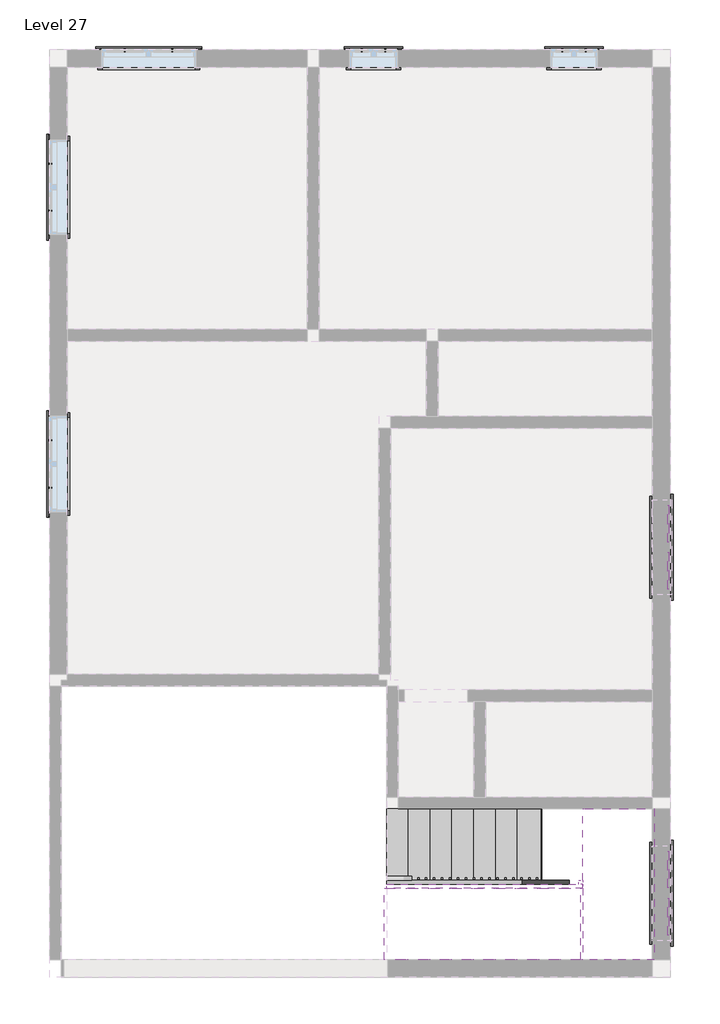
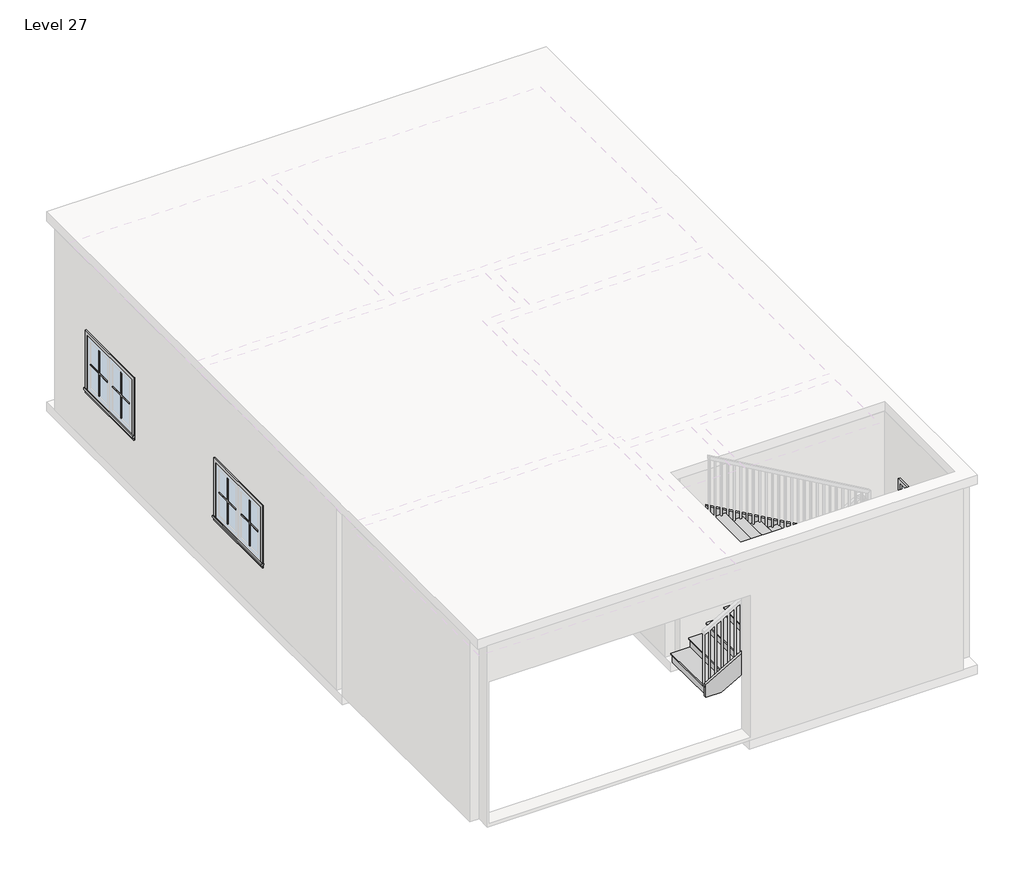
# One storey, part 3 of 3: 44 proxies, 6 members, 4 stair flights, 2 slabs.
"""IFC4 building model written with IfcOpenShell, lengths in millimetres."""

from ifc_helpers import new_model, si_unit, frame, origin, place, context, project, spatial, polyline, outline, extrude, transform, mapped, element, save
from components import muntin_pattern_2x2_muntin_pattern_2x2_2357e71d, muntin_pattern_2x2_muntin_pattern_2x2_302d8f29, muntin_pattern_2x2_muntin_pattern_2x2_53152e2c, muntin_pattern_2x2_muntin_pattern_2x2_e8f3e573, trim_window_exterior_flat_with_sill_c4e67c73, trim_window_exterior_flat_with_sill_a665a915, trim_window_interior_flat_picture_frame_cf1733af, trim_window_interior_flat_picture_frame_d485c387, non_monolithic_landing_8fd7ddd1, stair_flight_a002e3d3, stair_flight_1fb61bbc

model = new_model("IFC4")

# Units and contexts
model_context = context("Model", 3, world=origin())
ifc_project = project(units=[si_unit("LENGTHUNIT", "METRE", prefix="MILLI")], contexts=[model_context])

# Site, building, storey
site = spatial("IfcSite", under=ifc_project)
building = spatial("IfcBuilding", under=site)
storey = spatial("IfcBuildingStorey", under=building, Name="Level 27", Elevation=22402.8)

# Proxies
placement = place(None, origin())
muntin_pattern_2x2_muntin_pattern_2x2_shape = muntin_pattern_2x2_muntin_pattern_2x2_2357e71d(model_context)
element("IfcBuildingElementProxy", 1, Name="Muntin Pattern_2x2 : Muntin Pattern_2x2", ObjectType="Muntin Pattern_2x2 : Muntin Pattern_2x2", at=placement, inside=storey, context=model_context, shape_type="MappedRepresentation", body=[
    mapped(muntin_pattern_2x2_muntin_pattern_2x2_shape, transform((-4942.3279463, 5897.3080275, 23387.05), x_axis=(1.0, 0.0, 0.0), y_axis=(0.0, 1.0, 0.0), z_axis=(0.0, 0.0, 1.0))),
])
element("IfcBuildingElementProxy", 2, Name="Muntin Pattern_2x2 : Muntin Pattern_2x2", ObjectType="Muntin Pattern_2x2 : Muntin Pattern_2x2", at=placement, inside=storey, context=model_context, shape_type="MappedRepresentation", body=[
    mapped(muntin_pattern_2x2_muntin_pattern_2x2_shape, transform((-5899.5904463, 3838.3205275, 23387.05), x_axis=(0.0, 1.0, 0.0), y_axis=(-1.0, 0.0, 0.0), z_axis=(0.0, 0.0, 1.0))),
])
element("IfcBuildingElementProxy", 3, Name="Muntin Pattern_2x2 : Muntin Pattern_2x2", ObjectType="Muntin Pattern_2x2 : Muntin Pattern_2x2", at=placement, inside=storey, context=model_context, shape_type="MappedRepresentation", body=[
    mapped(muntin_pattern_2x2_muntin_pattern_2x2_shape, transform((-5899.5904463, 293.4330275, 23387.05), x_axis=(0.0, 1.0, 0.0), y_axis=(-1.0, 0.0, 0.0), z_axis=(0.0, 0.0, 1.0))),
])
element("IfcBuildingElementProxy", 4, Name="Muntin Pattern_2x2 : Muntin Pattern_2x2", ObjectType="Muntin Pattern_2x2 : Muntin Pattern_2x2", at=placement, inside=storey, context=model_context, shape_type="MappedRepresentation", body=[
    mapped(muntin_pattern_2x2_muntin_pattern_2x2_shape, transform((2031.5595537, -166.9419725, 23691.85), x_axis=(0.0, -1.0, 0.0), y_axis=(1.0, 0.0, 0.0), z_axis=(0.0, 0.0, 1.0))),
])
element("IfcBuildingElementProxy", 5, Name="Muntin Pattern_2x2 : Muntin Pattern_2x2", ObjectType="Muntin Pattern_2x2 : Muntin Pattern_2x2", at=placement, inside=storey, context=model_context, shape_type="MappedRepresentation", body=[
    mapped(muntin_pattern_2x2_muntin_pattern_2x2_shape, transform((2031.5595537, -4599.2419725, 23691.85), x_axis=(0.0, -1.0, 0.0), y_axis=(1.0, 0.0, 0.0), z_axis=(0.0, 0.0, 1.0))),
])
element("IfcBuildingElementProxy", 6, Name="Muntin Pattern_2x2 : Muntin Pattern_2x2", ObjectType="Muntin Pattern_2x2 : Muntin Pattern_2x2", at=placement, inside=storey, context=model_context, shape_type="MappedRepresentation", body=[
    mapped(muntin_pattern_2x2_muntin_pattern_2x2_shape, transform((-4942.3279463, 5897.3080275, 23387.05), x_axis=(1.0, 0.0, 0.0), y_axis=(0.0, 1.0, 0.0), z_axis=(0.0, 0.0, 1.0))),
])
element("IfcBuildingElementProxy", 7, Name="Muntin Pattern_2x2 : Muntin Pattern_2x2", ObjectType="Muntin Pattern_2x2 : Muntin Pattern_2x2", at=placement, inside=storey, context=model_context, shape_type="MappedRepresentation", body=[
    mapped(muntin_pattern_2x2_muntin_pattern_2x2_shape, transform((2031.5595537, -4599.2419725, 23691.85), x_axis=(0.0, -1.0, 0.0), y_axis=(1.0, 0.0, 0.0), z_axis=(0.0, 0.0, 1.0))),
])
muntin_pattern_2x2_muntin_pattern_2x2_2_shape = muntin_pattern_2x2_muntin_pattern_2x2_302d8f29(model_context)
element("IfcBuildingElementProxy", 8, Name="Muntin Pattern_2x2 : Muntin Pattern_2x2", ObjectType="Muntin Pattern_2x2 : Muntin Pattern_2x2", at=placement, inside=storey, context=model_context, shape_type="MappedRepresentation", body=[
    mapped(muntin_pattern_2x2_muntin_pattern_2x2_2_shape, transform((-4335.9029463, 5897.3080275, 23387.05), x_axis=(-1.0, 0.0, 0.0), y_axis=(0.0, -1.0, 0.0), z_axis=(0.0, 0.0, 1.0))),
])
element("IfcBuildingElementProxy", 9, Name="Muntin Pattern_2x2 : Muntin Pattern_2x2", ObjectType="Muntin Pattern_2x2 : Muntin Pattern_2x2", at=placement, inside=storey, context=model_context, shape_type="MappedRepresentation", body=[
    mapped(muntin_pattern_2x2_muntin_pattern_2x2_2_shape, transform((-5899.5904463, 4444.7455275, 23387.05), x_axis=(0.0, -1.0, 0.0), y_axis=(1.0, 0.0, 0.0), z_axis=(0.0, 0.0, 1.0))),
])
element("IfcBuildingElementProxy", 10, Name="Muntin Pattern_2x2 : Muntin Pattern_2x2", ObjectType="Muntin Pattern_2x2 : Muntin Pattern_2x2", at=placement, inside=storey, context=model_context, shape_type="MappedRepresentation", body=[
    mapped(muntin_pattern_2x2_muntin_pattern_2x2_2_shape, transform((-5899.5904463, 899.8580275, 23387.05), x_axis=(0.0, -1.0, 0.0), y_axis=(1.0, 0.0, 0.0), z_axis=(0.0, 0.0, 1.0))),
])
element("IfcBuildingElementProxy", 11, Name="Muntin Pattern_2x2 : Muntin Pattern_2x2", ObjectType="Muntin Pattern_2x2 : Muntin Pattern_2x2", at=placement, inside=storey, context=model_context, shape_type="MappedRepresentation", body=[
    mapped(muntin_pattern_2x2_muntin_pattern_2x2_2_shape, transform((2031.5595537, -773.3669725, 23691.85), x_axis=(0.0, 1.0, 0.0), y_axis=(-1.0, 0.0, 0.0), z_axis=(0.0, 0.0, 1.0))),
])
element("IfcBuildingElementProxy", 12, Name="Muntin Pattern_2x2 : Muntin Pattern_2x2", ObjectType="Muntin Pattern_2x2 : Muntin Pattern_2x2", at=placement, inside=storey, context=model_context, shape_type="MappedRepresentation", body=[
    mapped(muntin_pattern_2x2_muntin_pattern_2x2_2_shape, transform((2031.5595537, -5205.6669725, 23691.85), x_axis=(0.0, 1.0, 0.0), y_axis=(-1.0, 0.0, 0.0), z_axis=(0.0, 0.0, 1.0))),
])
element("IfcBuildingElementProxy", 13, Name="Muntin Pattern_2x2 : Muntin Pattern_2x2", ObjectType="Muntin Pattern_2x2 : Muntin Pattern_2x2", at=placement, inside=storey, context=model_context, shape_type="MappedRepresentation", body=[
    mapped(muntin_pattern_2x2_muntin_pattern_2x2_2_shape, transform((-4335.9029463, 5897.3080275, 23387.05), x_axis=(-1.0, 0.0, 0.0), y_axis=(0.0, -1.0, 0.0), z_axis=(0.0, 0.0, 1.0))),
])
element("IfcBuildingElementProxy", 14, Name="Muntin Pattern_2x2 : Muntin Pattern_2x2", ObjectType="Muntin Pattern_2x2 : Muntin Pattern_2x2", at=placement, inside=storey, context=model_context, shape_type="MappedRepresentation", body=[
    mapped(muntin_pattern_2x2_muntin_pattern_2x2_2_shape, transform((2031.5595537, -5205.6669725, 23691.85), x_axis=(0.0, 1.0, 0.0), y_axis=(-1.0, 0.0, 0.0), z_axis=(0.0, 0.0, 1.0))),
])
muntin_pattern_2x2_muntin_pattern_2x2_3_shape = muntin_pattern_2x2_muntin_pattern_2x2_53152e2c(model_context)
element("IfcBuildingElementProxy", 15, Name="Muntin Pattern_2x2 : Muntin Pattern_2x2", ObjectType="Muntin Pattern_2x2 : Muntin Pattern_2x2", at=placement, inside=storey, context=model_context, shape_type="MappedRepresentation", body=[
    mapped(muntin_pattern_2x2_muntin_pattern_2x2_3_shape, transform((-1907.0279463, 5897.3080275, 23387.05), x_axis=(1.0, 0.0, 0.0), y_axis=(0.0, 1.0, 0.0), z_axis=(0.0, 0.0, 1.0))),
])
element("IfcBuildingElementProxy", 16, Name="Muntin Pattern_2x2 : Muntin Pattern_2x2", ObjectType="Muntin Pattern_2x2 : Muntin Pattern_2x2", at=placement, inside=storey, context=model_context, shape_type="MappedRepresentation", body=[
    mapped(muntin_pattern_2x2_muntin_pattern_2x2_3_shape, transform((658.3720537, 5897.3080275, 23387.05), x_axis=(1.0, 0.0, 0.0), y_axis=(0.0, 1.0, 0.0), z_axis=(0.0, 0.0, 1.0))),
])
element("IfcBuildingElementProxy", 17, Name="Muntin Pattern_2x2 : Muntin Pattern_2x2", ObjectType="Muntin Pattern_2x2 : Muntin Pattern_2x2", at=placement, inside=storey, context=model_context, shape_type="MappedRepresentation", body=[
    mapped(muntin_pattern_2x2_muntin_pattern_2x2_3_shape, transform((-1907.0279463, 5897.3080275, 23387.05), x_axis=(1.0, 0.0, 0.0), y_axis=(0.0, 1.0, 0.0), z_axis=(0.0, 0.0, 1.0))),
])
element("IfcBuildingElementProxy", 18, Name="Muntin Pattern_2x2 : Muntin Pattern_2x2", ObjectType="Muntin Pattern_2x2 : Muntin Pattern_2x2", at=placement, inside=storey, context=model_context, shape_type="MappedRepresentation", body=[
    mapped(muntin_pattern_2x2_muntin_pattern_2x2_3_shape, transform((658.3720537, 5897.3080275, 23387.05), x_axis=(1.0, 0.0, 0.0), y_axis=(0.0, 1.0, 0.0), z_axis=(0.0, 0.0, 1.0))),
])
muntin_pattern_2x2_muntin_pattern_2x2_4_shape = muntin_pattern_2x2_muntin_pattern_2x2_e8f3e573(model_context)
element("IfcBuildingElementProxy", 19, Name="Muntin Pattern_2x2 : Muntin Pattern_2x2", ObjectType="Muntin Pattern_2x2 : Muntin Pattern_2x2", at=placement, inside=storey, context=model_context, shape_type="MappedRepresentation", body=[
    mapped(muntin_pattern_2x2_muntin_pattern_2x2_4_shape, transform((-1605.4029463, 5897.3080275, 23387.05), x_axis=(-1.0, 0.0, 0.0), y_axis=(0.0, -1.0, 0.0), z_axis=(0.0, 0.0, 1.0))),
])
element("IfcBuildingElementProxy", 20, Name="Muntin Pattern_2x2 : Muntin Pattern_2x2", ObjectType="Muntin Pattern_2x2 : Muntin Pattern_2x2", at=placement, inside=storey, context=model_context, shape_type="MappedRepresentation", body=[
    mapped(muntin_pattern_2x2_muntin_pattern_2x2_4_shape, transform((959.9970537, 5897.3080275, 23387.05), x_axis=(-1.0, 0.0, 0.0), y_axis=(0.0, -1.0, 0.0), z_axis=(0.0, 0.0, 1.0))),
])
element("IfcBuildingElementProxy", 21, Name="Muntin Pattern_2x2 : Muntin Pattern_2x2", ObjectType="Muntin Pattern_2x2 : Muntin Pattern_2x2", at=placement, inside=storey, context=model_context, shape_type="MappedRepresentation", body=[
    mapped(muntin_pattern_2x2_muntin_pattern_2x2_4_shape, transform((-1605.4029463, 5897.3080275, 23387.05), x_axis=(-1.0, 0.0, 0.0), y_axis=(0.0, -1.0, 0.0), z_axis=(0.0, 0.0, 1.0))),
])
element("IfcBuildingElementProxy", 22, Name="Muntin Pattern_2x2 : Muntin Pattern_2x2", ObjectType="Muntin Pattern_2x2 : Muntin Pattern_2x2", at=placement, inside=storey, context=model_context, shape_type="MappedRepresentation", body=[
    mapped(muntin_pattern_2x2_muntin_pattern_2x2_4_shape, transform((959.9970537, 5897.3080275, 23387.05), x_axis=(-1.0, 0.0, 0.0), y_axis=(0.0, -1.0, 0.0), z_axis=(0.0, 0.0, 1.0))),
])
trim_window_exterior_flat_with_sill_shape = trim_window_exterior_flat_with_sill_c4e67c73(model_context)
element("IfcBuildingElementProxy", 23, Name="Trim-Window-Exterior-Flat : with Sill", ObjectType="Trim-Window-Exterior-Flat : with Sill", at=placement, inside=storey, context=model_context, shape_type="MappedRepresentation", body=[
    mapped(trim_window_exterior_flat_with_sill_shape, transform((-4639.1154463, 5906.8330275, 24231.6), x_axis=(-1.0, 0.0, 0.0), y_axis=(0.0, 0.0, 1.0), z_axis=(0.0, 1.0, 0.0))),
])
element("IfcBuildingElementProxy", 24, Name="Trim-Window-Exterior-Flat : with Sill", ObjectType="Trim-Window-Exterior-Flat : with Sill", at=placement, inside=storey, context=model_context, shape_type="MappedRepresentation", body=[
    mapped(trim_window_exterior_flat_with_sill_shape, transform((-5909.1154463, 4141.5330275, 24231.6), x_axis=(0.0, -1.0, 0.0), y_axis=(0.0, 0.0, 1.0), z_axis=(-1.0, 0.0, 0.0))),
])
element("IfcBuildingElementProxy", 25, Name="Trim-Window-Exterior-Flat : with Sill", ObjectType="Trim-Window-Exterior-Flat : with Sill", at=placement, inside=storey, context=model_context, shape_type="MappedRepresentation", body=[
    mapped(trim_window_exterior_flat_with_sill_shape, transform((-5909.1154463, 596.6455275, 24231.6), x_axis=(0.0, -1.0, 0.0), y_axis=(0.0, 0.0, 1.0), z_axis=(-1.0, 0.0, 0.0))),
])
element("IfcBuildingElementProxy", 26, Name="Trim-Window-Exterior-Flat : with Sill", ObjectType="Trim-Window-Exterior-Flat : with Sill", at=placement, inside=storey, context=model_context, shape_type="MappedRepresentation", body=[
    mapped(trim_window_exterior_flat_with_sill_shape, transform((2041.0845537, -470.1544725, 24536.4), x_axis=(0.0, 1.0, 0.0), y_axis=(0.0, 0.0, 1.0), z_axis=(1.0, 0.0, 0.0))),
])
element("IfcBuildingElementProxy", 27, Name="Trim-Window-Exterior-Flat : with Sill", ObjectType="Trim-Window-Exterior-Flat : with Sill", at=placement, inside=storey, context=model_context, shape_type="MappedRepresentation", body=[
    mapped(trim_window_exterior_flat_with_sill_shape, transform((2041.0845537, -4902.4544725, 24536.4), x_axis=(0.0, 1.0, 0.0), y_axis=(0.0, 0.0, 1.0), z_axis=(1.0, 0.0, 0.0))),
])
element("IfcBuildingElementProxy", 28, Name="Trim-Window-Exterior-Flat : with Sill", ObjectType="Trim-Window-Exterior-Flat : with Sill", at=placement, inside=storey, context=model_context, shape_type="MappedRepresentation", body=[
    mapped(trim_window_exterior_flat_with_sill_shape, transform((-4639.1154463, 5906.8330275, 24231.6), x_axis=(-1.0, 0.0, 0.0), y_axis=(0.0, 0.0, 1.0), z_axis=(0.0, 1.0, 0.0))),
])
element("IfcBuildingElementProxy", 29, Name="Trim-Window-Exterior-Flat : with Sill", ObjectType="Trim-Window-Exterior-Flat : with Sill", at=placement, inside=storey, context=model_context, shape_type="MappedRepresentation", body=[
    mapped(trim_window_exterior_flat_with_sill_shape, transform((2041.0845537, -4902.4544725, 24536.4), x_axis=(0.0, 1.0, 0.0), y_axis=(0.0, 0.0, 1.0), z_axis=(1.0, 0.0, 0.0))),
])
trim_window_exterior_flat_with_sill_2_shape = trim_window_exterior_flat_with_sill_a665a915(model_context)
element("IfcBuildingElementProxy", 30, Name="Trim-Window-Exterior-Flat : with Sill", ObjectType="Trim-Window-Exterior-Flat : with Sill", at=placement, inside=storey, context=model_context, shape_type="MappedRepresentation", body=[
    mapped(trim_window_exterior_flat_with_sill_2_shape, transform((-1756.2154463, 5906.8330275, 24231.6), x_axis=(-1.0, 0.0, 0.0), y_axis=(0.0, 0.0, 1.0), z_axis=(0.0, 1.0, 0.0))),
])
element("IfcBuildingElementProxy", 31, Name="Trim-Window-Exterior-Flat : with Sill", ObjectType="Trim-Window-Exterior-Flat : with Sill", at=placement, inside=storey, context=model_context, shape_type="MappedRepresentation", body=[
    mapped(trim_window_exterior_flat_with_sill_2_shape, transform((809.1845537, 5906.8330275, 24231.6), x_axis=(-1.0, 0.0, 0.0), y_axis=(0.0, 0.0, 1.0), z_axis=(0.0, 1.0, 0.0))),
])
element("IfcBuildingElementProxy", 32, Name="Trim-Window-Exterior-Flat : with Sill", ObjectType="Trim-Window-Exterior-Flat : with Sill", at=placement, inside=storey, context=model_context, shape_type="MappedRepresentation", body=[
    mapped(trim_window_exterior_flat_with_sill_2_shape, transform((-1756.2154463, 5906.8330275, 24231.6), x_axis=(-1.0, 0.0, 0.0), y_axis=(0.0, 0.0, 1.0), z_axis=(0.0, 1.0, 0.0))),
])
element("IfcBuildingElementProxy", 33, Name="Trim-Window-Exterior-Flat : with Sill", ObjectType="Trim-Window-Exterior-Flat : with Sill", at=placement, inside=storey, context=model_context, shape_type="MappedRepresentation", body=[
    mapped(trim_window_exterior_flat_with_sill_2_shape, transform((809.1845537, 5906.8330275, 24231.6), x_axis=(-1.0, 0.0, 0.0), y_axis=(0.0, 0.0, 1.0), z_axis=(0.0, 1.0, 0.0))),
])
trim_window_interior_flat_picture_frame_shape = trim_window_interior_flat_picture_frame_cf1733af(model_context)
element("IfcBuildingElementProxy", 34, Name="Trim-Window-Interior-Flat : Picture Frame", ObjectType="Trim-Window-Interior-Flat : Picture Frame", at=placement, inside=storey, context=model_context, shape_type="MappedRepresentation", body=[
    mapped(trim_window_interior_flat_picture_frame_shape, transform((-4639.1154463, 5678.2330275, 24231.6), x_axis=(1.0, 0.0, 0.0), y_axis=(0.0, 0.0, 1.0), z_axis=(0.0, -1.0, 0.0))),
])
element("IfcBuildingElementProxy", 35, Name="Trim-Window-Interior-Flat : Picture Frame", ObjectType="Trim-Window-Interior-Flat : Picture Frame", at=placement, inside=storey, context=model_context, shape_type="MappedRepresentation", body=[
    mapped(trim_window_interior_flat_picture_frame_shape, transform((-5680.5154463, 4141.5330275, 24231.6), x_axis=(0.0, 1.0, 0.0), y_axis=(0.0, 0.0, 1.0), z_axis=(1.0, 0.0, 0.0))),
])
element("IfcBuildingElementProxy", 36, Name="Trim-Window-Interior-Flat : Picture Frame", ObjectType="Trim-Window-Interior-Flat : Picture Frame", at=placement, inside=storey, context=model_context, shape_type="MappedRepresentation", body=[
    mapped(trim_window_interior_flat_picture_frame_shape, transform((-5680.5154463, 596.6455275, 24231.6), x_axis=(0.0, 1.0, 0.0), y_axis=(0.0, 0.0, 1.0), z_axis=(1.0, 0.0, 0.0))),
])
element("IfcBuildingElementProxy", 37, Name="Trim-Window-Interior-Flat : Picture Frame", ObjectType="Trim-Window-Interior-Flat : Picture Frame", at=placement, inside=storey, context=model_context, shape_type="MappedRepresentation", body=[
    mapped(trim_window_interior_flat_picture_frame_shape, transform((1812.4845537, -470.1544725, 24536.4), x_axis=(0.0, -1.0, 0.0), y_axis=(0.0, 0.0, 1.0), z_axis=(-1.0, 0.0, 0.0))),
])
element("IfcBuildingElementProxy", 38, Name="Trim-Window-Interior-Flat : Picture Frame", ObjectType="Trim-Window-Interior-Flat : Picture Frame", at=placement, inside=storey, context=model_context, shape_type="MappedRepresentation", body=[
    mapped(trim_window_interior_flat_picture_frame_shape, transform((1812.4845537, -4902.4544725, 24536.4), x_axis=(0.0, -1.0, 0.0), y_axis=(0.0, 0.0, 1.0), z_axis=(-1.0, 0.0, 0.0))),
])
element("IfcBuildingElementProxy", 39, Name="Trim-Window-Interior-Flat : Picture Frame", ObjectType="Trim-Window-Interior-Flat : Picture Frame", at=placement, inside=storey, context=model_context, shape_type="MappedRepresentation", body=[
    mapped(trim_window_interior_flat_picture_frame_shape, transform((-4639.1154463, 5678.2330275, 24231.6), x_axis=(1.0, 0.0, 0.0), y_axis=(0.0, 0.0, 1.0), z_axis=(0.0, -1.0, 0.0))),
])
element("IfcBuildingElementProxy", 40, Name="Trim-Window-Interior-Flat : Picture Frame", ObjectType="Trim-Window-Interior-Flat : Picture Frame", at=placement, inside=storey, context=model_context, shape_type="MappedRepresentation", body=[
    mapped(trim_window_interior_flat_picture_frame_shape, transform((1812.4845537, -4902.4544725, 24536.4), x_axis=(0.0, -1.0, 0.0), y_axis=(0.0, 0.0, 1.0), z_axis=(-1.0, 0.0, 0.0))),
])
trim_window_interior_flat_picture_frame_2_shape = trim_window_interior_flat_picture_frame_d485c387(model_context)
element("IfcBuildingElementProxy", 41, Name="Trim-Window-Interior-Flat : Picture Frame", ObjectType="Trim-Window-Interior-Flat : Picture Frame", at=placement, inside=storey, context=model_context, shape_type="MappedRepresentation", body=[
    mapped(trim_window_interior_flat_picture_frame_2_shape, transform((-1756.2154463, 5678.2330275, 24231.6), x_axis=(1.0, 0.0, 0.0), y_axis=(0.0, 0.0, 1.0), z_axis=(0.0, -1.0, 0.0))),
])
element("IfcBuildingElementProxy", 42, Name="Trim-Window-Interior-Flat : Picture Frame", ObjectType="Trim-Window-Interior-Flat : Picture Frame", at=placement, inside=storey, context=model_context, shape_type="MappedRepresentation", body=[
    mapped(trim_window_interior_flat_picture_frame_2_shape, transform((809.1845537, 5678.2330275, 24231.6), x_axis=(1.0, 0.0, 0.0), y_axis=(0.0, 0.0, 1.0), z_axis=(0.0, -1.0, 0.0))),
])
element("IfcBuildingElementProxy", 43, Name="Trim-Window-Interior-Flat : Picture Frame", ObjectType="Trim-Window-Interior-Flat : Picture Frame", at=placement, inside=storey, context=model_context, shape_type="MappedRepresentation", body=[
    mapped(trim_window_interior_flat_picture_frame_2_shape, transform((-1756.2154463, 5678.2330275, 24231.6), x_axis=(1.0, 0.0, 0.0), y_axis=(0.0, 0.0, 1.0), z_axis=(0.0, -1.0, 0.0))),
])
element("IfcBuildingElementProxy", 44, Name="Trim-Window-Interior-Flat : Picture Frame", ObjectType="Trim-Window-Interior-Flat : Picture Frame", at=placement, inside=storey, context=model_context, shape_type="MappedRepresentation", body=[
    mapped(trim_window_interior_flat_picture_frame_2_shape, transform((809.1845537, 5678.2330275, 24231.6), x_axis=(1.0, 0.0, 0.0), y_axis=(0.0, 0.0, 1.0), z_axis=(0.0, -1.0, 0.0))),
])

# Members
element("IfcMember", 45, ObjectType="Stringer - 2\" Width", at=placement, inside=storey, context=model_context, shape_type="SweptSolid", body=[
    extrude(outline(polyline([(22611.8890626, -1591.1154463), (22402.8, -1591.1154463), (22402.8, -1342.8974141), (23671.724218, 872.6845537), (24022.9745172, 872.6845537), (22611.8890626, -1591.1154463)])), frame((0.0, -4788.1544725, 0.0), z_axis=(0.0, 1.0, 0.0), x_axis=(0.0, 0.0, 1.0)), (0.0, 0.0, 1.0), 50.8),
])
element("IfcMember", 46, ObjectType="Stringer - 2\" Width", at=placement, inside=storey, context=model_context, shape_type="SweptSolid", body=[
    extrude(outline(polyline([(23860.8387634, 923.4845537), (24212.0890626, 923.4845537), (25652.2690626, -1591.1154463), (25301.0187634, -1591.1154463), (23860.8387634, 923.4845537)])), frame((0.0, -4838.9544725, 0.0), z_axis=(0.0, 1.0, 0.0), x_axis=(0.0, 0.0, 1.0)), (0.0, 0.0, 1.0), 50.8),
])
element("IfcMember", 47, ObjectType="Stringer - 2\" Width", at=placement, inside=storey, context=model_context, shape_type="SweptSolid", body=[
    extrude(outline(polyline([(872.6845537, -4737.3544725), (923.4845537, -4737.3544725), (923.4845537, -4788.1544725), (872.6845537, -4788.1544725), (872.6845537, -4737.3544725)])), frame((0.0, 0.0, 23774.4), z_axis=(0.0, 0.0, 1.0), x_axis=(1.0, 0.0, 0.0)), (0.0, 0.0, 1.0), 304.8),
])
element("IfcMember", 48, ObjectType="Stringer - 2\" Width", at=placement, inside=storey, context=model_context, shape_type="SweptSolid", body=[
    extrude(outline(polyline([(22611.8890626, -1591.1154463), (22402.8, -1591.1154463), (22402.8, -1342.8974141), (23671.724218, 872.6845537), (24022.9745172, 872.6845537), (22611.8890626, -1591.1154463)])), frame((0.0, -4788.1544725, 0.0), z_axis=(0.0, 1.0, 0.0), x_axis=(0.0, 0.0, 1.0)), (0.0, 0.0, 1.0), 50.8),
])
element("IfcMember", 49, ObjectType="Stringer - 2\" Width", at=placement, inside=storey, context=model_context, shape_type="SweptSolid", body=[
    extrude(outline(polyline([(23860.8387634, 923.4845537), (24212.0890626, 923.4845537), (25652.2690626, -1591.1154463), (25301.0187634, -1591.1154463), (23860.8387634, 923.4845537)])), frame((0.0, -4838.9544725, 0.0), z_axis=(0.0, 1.0, 0.0), x_axis=(0.0, 0.0, 1.0)), (0.0, 0.0, 1.0), 50.8),
])
element("IfcMember", 50, ObjectType="Stringer - 2\" Width", at=placement, inside=storey, context=model_context, shape_type="SweptSolid", body=[
    extrude(outline(polyline([(872.6845537, -4737.3544725), (923.4845537, -4737.3544725), (923.4845537, -4788.1544725), (872.6845537, -4788.1544725), (872.6845537, -4737.3544725)])), frame((0.0, 0.0, 23774.4), z_axis=(0.0, 0.0, 1.0), x_axis=(1.0, 0.0, 0.0)), (0.0, 0.0, 1.0), 304.8),
])

# Slabs
non_monolithic_landing_shape = non_monolithic_landing_8fd7ddd1(model_context)
element("IfcSlab", 51, ObjectType="Non-Monolithic Landing", at=placement, inside=storey, context=model_context, shape_type="MappedRepresentation", body=[
    mapped(non_monolithic_landing_shape, transform((0.0, 0.0, 0.0), x_axis=(1.0, 0.0, 0.0), y_axis=(0.0, 1.0, 0.0), z_axis=(0.0, 0.0, 1.0))),
])
element("IfcSlab", 52, ObjectType="Non-Monolithic Landing", at=placement, inside=storey, context=model_context, shape_type="MappedRepresentation", body=[
    mapped(non_monolithic_landing_shape, transform((0.0, 0.0, 0.0), x_axis=(1.0, 0.0, 0.0), y_axis=(0.0, 1.0, 0.0), z_axis=(0.0, 0.0, 1.0))),
])

# Stair flights
stair_flight_shape = stair_flight_a002e3d3(model_context)
element("IfcStairFlight", 53, ObjectType="2\" Tread 1\" Nosing 1/4\" Riser", at=placement, inside=storey, context=model_context, shape_type="MappedRepresentation", body=[
    mapped(stair_flight_shape, transform((0.0, 0.0, 0.0), x_axis=(1.0, 0.0, 0.0), y_axis=(0.0, 1.0, 0.0), z_axis=(0.0, 0.0, 1.0))),
])
stair_flight_2_shape = stair_flight_1fb61bbc(model_context)
element("IfcStairFlight", 54, ObjectType="2\" Tread 1\" Nosing 1/4\" Riser", at=placement, inside=storey, context=model_context, shape_type="MappedRepresentation", body=[
    mapped(stair_flight_2_shape, transform((0.0, 0.0, 0.0), x_axis=(1.0, 0.0, 0.0), y_axis=(0.0, 1.0, 0.0), z_axis=(0.0, 0.0, 1.0))),
])
element("IfcStairFlight", 55, ObjectType="2\" Tread 1\" Nosing 1/4\" Riser", at=placement, inside=storey, context=model_context, shape_type="MappedRepresentation", body=[
    mapped(stair_flight_shape, transform((0.0, 0.0, 0.0), x_axis=(1.0, 0.0, 0.0), y_axis=(0.0, 1.0, 0.0), z_axis=(0.0, 0.0, 1.0))),
])
element("IfcStairFlight", 56, ObjectType="2\" Tread 1\" Nosing 1/4\" Riser", at=placement, inside=storey, context=model_context, shape_type="MappedRepresentation", body=[
    mapped(stair_flight_2_shape, transform((0.0, 0.0, 0.0), x_axis=(1.0, 0.0, 0.0), y_axis=(0.0, 1.0, 0.0), z_axis=(0.0, 0.0, 1.0))),
])

save(model, "model.ifc")

# Revit data of these elements
# Type "Muntin Pattern_2x2 : Muntin Pattern_2x2"
#   Width [instance default] = 4' - 0"
#   Thickness = 0' - 0 1/2"
#   Height [instance default] = 4' - 0"
#   Distance = 0' - 0 3/4"
#   Interior Material [instance default] = none
#   Exterior Material [instance default] = none
#   Default Elevation = 0
# Type "Trim-Window-Exterior-Flat : with Sill"
#   Trim Width = 0' - 2 1/4"
#   Trim Thickness_Picture Frame = 0' - 1 1/4"
#   Trim Thickness_with Sill = 0' - 0 3/4"
#   Sill Thickness = 0' - 1 1/4"
#   Opening Width [instance default] = 2' - 0"
#   Opening Height [instance default] = 3' - 0"
#   Default Elevation = 4' - 0"
#   Sill = yes
#   Picture Frame = no
#   Trim Material [instance default] = none
# Type "Trim-Window-Interior-Flat : Picture Frame"
#   Trim Thickness_Picture Frame = 0' - 1 1/4"
#   Trim Width = 0' - 2 1/4"
#   Trim Thickness_with Sill = 0' - 0 3/4"
#   Sill Thickness = 0' - 1 1/4"
#   Opening Width [instance default] = 2' - 0"
#   Opening Height [instance default] = 3' - 0"
#   Default Elevation = 4' - 0"
#   Sill = no
#   Picture Frame = yes
#   Trim Material [instance default] = none
# Elements 1, 2, 3, 4, 5, 6, 7, 8, 9, 10, 11, 12, 13, 14 (IfcBuildingElementProxy, "Muntin Pattern_2x2 : Muntin Pattern_2x2")
#   Width = 1' - 6 5/8"
#   Height = 2' - 6 1/2"
#   Interior Material = Wood - Stained
#   Exterior Material = Clad - White
#   Phase Created = New Construction
#   Materials on its faces: "Clad - White", "Wood - Stained"
# Elements 15, 16, 17, 18, 19, 20, 21, 22 (IfcBuildingElementProxy, "Muntin Pattern_2x2 : Muntin Pattern_2x2")
#   Width = 0' - 6 5/8"
#   Height = 2' - 6 1/2"
#   Interior Material = Wood - Stained
#   Exterior Material = Clad - White
#   Phase Created = New Construction
#   Materials on its faces: "Clad - White", "Wood - Stained"
# Elements 23, 24, 25, 26, 27, 28, 29 (IfcBuildingElementProxy, "Trim-Window-Exterior-Flat : with Sill")
#   Opening Width = 4' - 0"
#   Opening Height = 3' - 0"
#   Trim Material = Clad - White
#   Phase Created = New Construction
#   Materials on its faces: "Clad - White"
# Elements 30, 31, 32, 33 (IfcBuildingElementProxy, "Trim-Window-Exterior-Flat : with Sill")
#   Opening Width = 2' - 0"
#   Opening Height = 3' - 0"
#   Trim Material = Clad - White
#   Phase Created = New Construction
#   Materials on its faces: "Clad - White"
# Elements 34, 35, 36, 37, 38, 39, 40 (IfcBuildingElementProxy, "Trim-Window-Interior-Flat : Picture Frame")
#   Opening Width = 4' - 0"
#   Opening Height = 3' - 0"
#   Trim Material = Wood - Stained
#   Phase Created = New Construction
#   Materials on its faces: "Wood - Stained"
# Elements 41, 42, 43, 44 (IfcBuildingElementProxy, "Trim-Window-Interior-Flat : Picture Frame")
#   Opening Width = 2' - 0"
#   Opening Height = 3' - 0"
#   Trim Material = Wood - Stained
#   Phase Created = New Construction
#   Materials on its faces: "Wood - Stained"
# Elements 45, 46, 47, 48, 49, 50 (IfcMember, "Stringer - 2\" Width")
#   Phase Created = New Construction
# Elements 51, 52 (IfcSlab, "Non-Monolithic Landing")
#   Phase Created = New Construction
# Elements 53, 54, 55, 56 (IfcStairFlight, "2\" Tread 1\" Nosing 1/4\" Riser")
#   Phase Created = New Construction
# Materials
#   "Clad - White": class "Wood", colour RGB 242 242 238, transparency 0, Cost = 0
#   "Wood - Stained": class "Wood", colour RGB 224 178 126, transparency 0, Cost = 0
